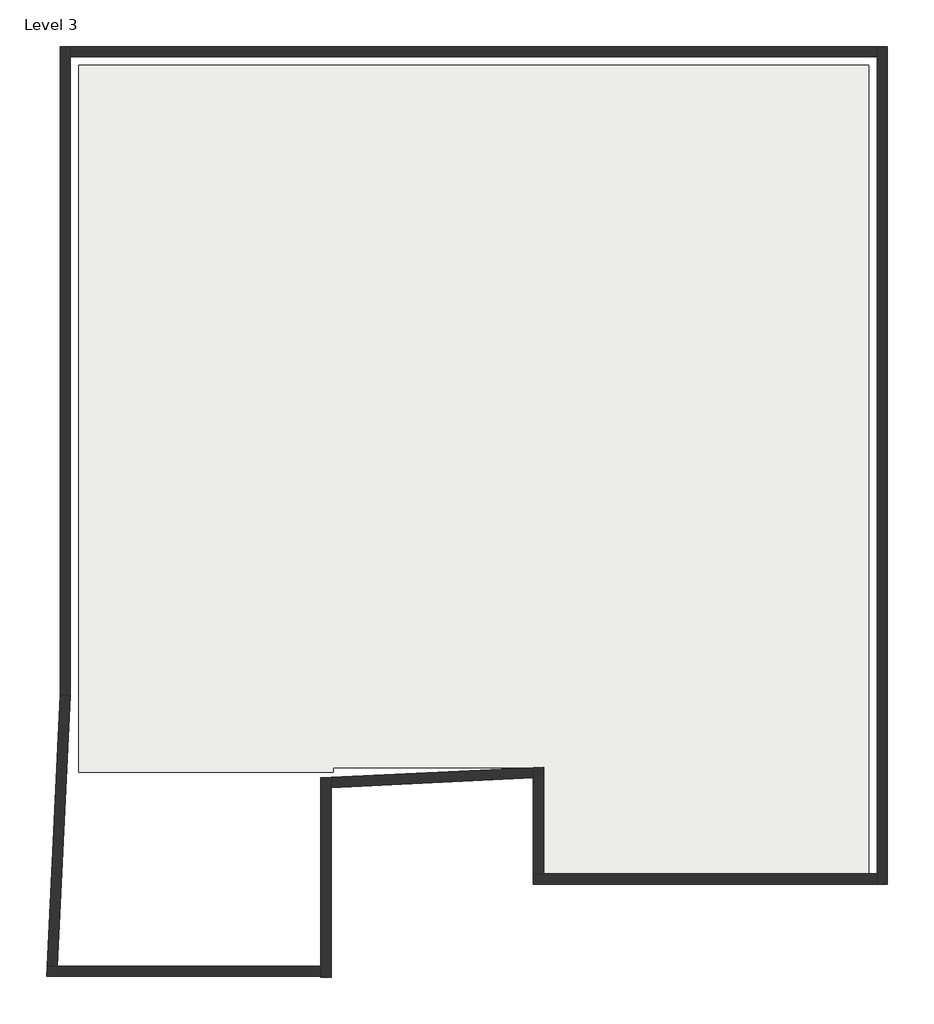
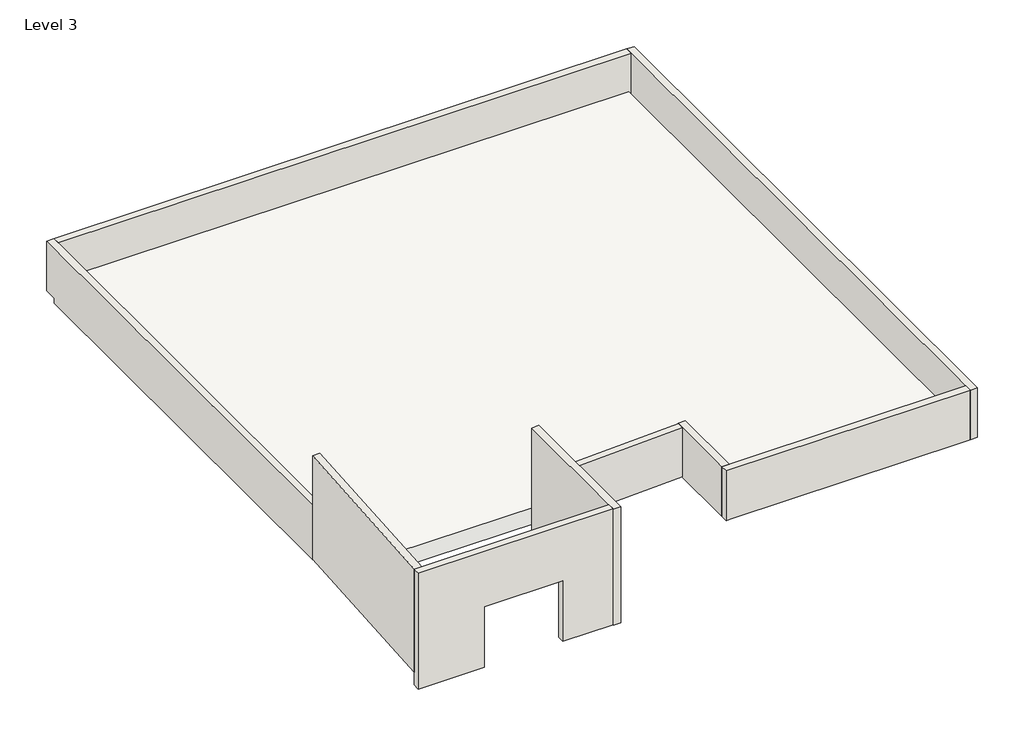
# One storey: 9 walls, 1 roof.
"""IFC4 building model written with IfcOpenShell, lengths in millimetres."""

from ifc_helpers import new_model, si_unit, frame, origin, place, context, project, spatial, polyline, outline, extrude, faceted_brep, element, save

model = new_model("IFC4")

# Units and contexts
model_context = context("Model", 3, world=origin())
ifc_project = project(units=[si_unit("LENGTHUNIT", "METRE", prefix="MILLI")], contexts=[model_context])

# Site, building, storey
site = spatial("IfcSite", under=ifc_project)
building = spatial("IfcBuilding", under=site)
storey = spatial("IfcBuildingStorey", under=building, Name="Level 3", Elevation=6400.8)

# Roof
placement = place(None, origin())
element("IfcRoof", 1, ObjectType="Generic - 12\"", at=placement, inside=storey, context=model_context, shape_type="SweptSolid", body=[
    extrude(outline(polyline([(-14760.7023867, 8292.2500137), (-4981.7023867, 8292.2500137), (-4981.7023867, -1718.5249863), (-9071.1023867, -1718.5249863), (-9071.1023867, -400.8999863), (-11611.1023867, -400.8999863), (-11611.1023867, -458.0499863), (-14760.7023867, -458.0499863), (-14760.7023867, 8292.2500137)])), frame((0.0, 0.0, 6705.6), z_axis=(0.0, 0.0, 1.0), x_axis=(1.0, 0.0, 0.0)), (0.0, 0.0, 1.0), 304.8),
])

# Walls
element("IfcWall", 2, ObjectType="INNER WALL 5\"", at=placement, inside=storey, context=model_context, shape_type="SweptSolid", body=[
    extrude(outline(polyline([(-4880.1023867, 8393.8500137), (-14863.8898867, 8393.8500137), (-14863.8898867, 8520.8500137), (-4880.1023867, 8520.8500137), (-4880.1023867, 8393.8500137)])), frame((0.0, 0.0, 6705.6), z_axis=(0.0, 0.0, 1.0), x_axis=(1.0, 0.0, 0.0)), (0.0, 0.0, 1.0), 914.4),
])
element("IfcWall", 3, ObjectType="INNER WALL 5\"", at=placement, inside=storey, context=model_context, shape_type="Brep", body=[
    faceted_brep([(-4753.1023867, -1842.3499863, 6705.6), (-4753.1023867, 8292.2500137, 6705.6), (-4753.1023867, 8520.8500137, 6705.6), (-4753.1023867, 8520.8500137, 7620.0), (-4753.1023867, -1842.3499863, 7620.0), (-4880.1023867, -1842.3499863, 6705.6), (-4880.1023867, -1842.3499863, 7620.0), (-4880.1023867, -1715.3499863, 7620.0), (-4880.1023867, 8393.8500137, 7620.0), (-4880.1023867, 8520.8500137, 7620.0), (-4880.1023867, 8520.8500137, 6705.6), (-4880.1023867, 8393.8500137, 6705.6), (-4880.1023867, -1715.3499863, 6705.6)], [[[0, 1, 2, 3, 4]], [[5, 6, 7, 8, 9, 10, 11, 12]], [[2, 1, 0, 5, 12, 11, 10]], [[4, 3, 9, 8, 7, 6]], [[3, 2, 10, 9]], [[0, 4, 6, 5]]]),
])
element("IfcWall", 4, ObjectType="INNER WALL 5\"", at=placement, inside=storey, context=model_context, shape_type="Brep", body=[
    faceted_brep([(-14990.8898867, 8292.2500137, 6618.3549278), (-14990.8898867, 492.69606, 6618.3549278), (-14990.8898867, 492.69606, 7620.0), (-14990.8898867, 8520.8500137, 7620.0), (-14990.8898867, 8520.8500137, 6705.6), (-14990.8898867, 8292.2500137, 6705.6), (-14863.8898867, 8292.2500137, 6618.3549278), (-14863.8898867, 8292.2500137, 6705.6), (-14863.8898867, 8393.8500137, 6705.6), (-14863.8898867, 8520.8500137, 6705.6), (-14863.8898867, 8520.8500137, 7620.0), (-14863.8898867, 8393.8500137, 7620.0), (-14863.8898867, 489.6542677, 7620.0), (-14863.8898867, 489.6542677, 6618.3549278)], [[[0, 1, 2, 3, 4, 5]], [[6, 7, 8, 9, 10, 11, 12, 13]], [[1, 0, 6, 13]], [[3, 2, 12, 11, 10]], [[4, 9, 8, 7, 5]], [[0, 5, 7, 6]], [[4, 3, 10, 9]], [[2, 1, 13, 12]]]),
])
element("IfcWall", 5, ObjectType="INNER WALL 5\"", at=placement, inside=storey, context=model_context, shape_type="Brep", body=[
    faceted_brep([(-11763.5023867, -2985.3499863, 8534.4), (-15157.5917172, -2985.3499863, 8534.4), (-15157.5917172, -2985.3499863, 6400.8), (-14011.4023867, -2985.3499863, 6400.8), (-14011.4023867, -2985.3499863, 7520.3640825), (-12639.8023867, -2985.3499863, 7520.3640825), (-12639.8023867, -2985.3499863, 6400.8), (-11763.5023867, -2985.3499863, 6400.8), (-15151.5046407, -2858.3499863, 8534.4), (-15024.3588484, -2858.3499863, 8534.4), (-11763.5023867, -2858.3499863, 8534.4), (-11763.5023867, -2858.3499863, 6400.8), (-12639.8023867, -2858.3499863, 6400.8), (-12639.8023867, -2858.3499863, 7520.3640825), (-14011.4023867, -2858.3499863, 7520.3640825), (-14011.4023867, -2858.3499863, 6400.8), (-15151.5046407, -2858.3499863, 6400.8), (-15151.5046407, -2858.3499863, 6630.8481004)], [[[0, 1, 2, 3, 4, 5, 6, 7]], [[8, 9, 10, 11, 12, 13, 14, 15, 16, 17]], [[11, 7, 6, 12]], [[2, 16, 15, 3]], [[1, 0, 10, 9, 8]], [[0, 7, 11, 10]], [[2, 1, 8, 17, 16]], [[5, 13, 12, 6]], [[13, 5, 4, 14]], [[14, 4, 3, 15]]]),
])
element("IfcWall", 6, ObjectType="INNER WALL 5\"", at=placement, inside=storey, context=model_context, shape_type="Brep", body=[
    faceted_brep([(-4880.1023867, -1715.3499863, 6705.6), (-4981.7023867, -1715.3499863, 6705.6), (-9007.6023867, -1715.3499863, 6705.6), (-9071.1023867, -1715.3499863, 6705.6), (-9134.6023867, -1715.3499863, 6705.6), (-9134.6023867, -1715.3499863, 7620.0), (-9007.6023867, -1715.3499863, 7620.0), (-4880.1023867, -1715.3499863, 7620.0), (-4880.1023867, -1842.3499863, 6705.6), (-4880.1023867, -1842.3499863, 7620.0), (-9134.6023867, -1842.3499863, 7620.0), (-9134.6023867, -1842.3499863, 6705.6), (-9071.1023867, -1842.3499863, 6705.6), (-4981.7023867, -1842.3499863, 6705.6)], [[[0, 1, 2, 3, 4, 5, 6, 7]], [[8, 9, 10, 11, 12, 13]], [[4, 3, 2, 1, 0, 8, 13, 12, 11]], [[7, 6, 5, 10, 9]], [[5, 4, 11, 10]], [[0, 7, 9, 8]]]),
])
element("IfcWall", 7, ObjectType="INNER WALL 5\"", at=placement, inside=storey, context=model_context, shape_type="Brep", body=[
    faceted_brep([(-9007.6023867, -1715.3499863, 6705.6), (-9007.6023867, -394.6969014, 6705.6), (-9007.6023867, -394.6969014, 7620.0), (-9007.6023867, -1715.3499863, 7620.0), (-9134.6023867, -1715.3499863, 6705.6), (-9134.6023867, -1715.3499863, 7620.0), (-9134.6023867, -400.8999863, 7620.0), (-9134.6023867, -400.8999863, 7618.4335882), (-9134.6023867, -400.8999863, 6713.109375), (-9134.6023867, -400.8999863, 6705.6)], [[[0, 1, 2, 3]], [[4, 5, 6, 7, 8, 9]], [[1, 0, 4, 9]], [[3, 2, 6, 5]], [[0, 3, 5, 4]], [[2, 1, 9, 8, 7, 6]]]),
])
element("IfcWall", 8, ObjectType="INNER WALL 5\"", at=placement, inside=storey, context=model_context, shape_type="Brep", body=[
    faceted_brep([(-11636.5023867, -2998.0499863, 6400.8), (-11636.5023867, -523.1007575, 6400.8), (-11636.5023867, -523.1007575, 6713.109375), (-11636.5023867, -523.1007575, 7618.4335882), (-11636.5023867, -523.1007575, 8534.4), (-11636.5023867, -2998.0499863, 8534.4), (-11763.5023867, -2998.0499863, 6400.8), (-11763.5023867, -2998.0499863, 8534.4), (-11763.5023867, -2985.3499863, 8534.4), (-11763.5023867, -2858.3499863, 8534.4), (-11763.5023867, -529.3038423, 8534.4), (-11763.5023867, -529.3038423, 6400.8), (-11763.5023867, -2858.3499863, 6400.8), (-11763.5023867, -2985.3499863, 6400.8)], [[[0, 1, 2, 3, 4, 5]], [[6, 7, 8, 9, 10, 11, 12, 13]], [[1, 0, 6, 13, 12, 11]], [[5, 4, 10, 9, 8, 7]], [[0, 5, 7, 6]], [[4, 3, 2, 1, 11, 10]]]),
])
element("IfcWall", 9, ObjectType="INNER WALL 5\"", at=placement, inside=storey, context=model_context, shape_type="SweptSolid", body=[
    extrude(outline(polyline([(-14863.8898867, 489.6542677), (-15024.3588484, -2858.3499863), (-15151.5046407, -2858.3499863), (-14990.8898867, 492.69606), (-14863.8898867, 489.6542677)])), frame((0.0, 0.0, 6630.8481004), z_axis=(0.0, 0.0, 1.0), x_axis=(1.0, 0.0, 0.0)), (0.0, 0.0, 1.0), 1903.5518996),
])
element("IfcWall", 10, ObjectType="INNER WALL 5\"", at=placement, inside=storey, context=model_context, shape_type="SweptSolid", body=[
    extrude(outline(polyline([(-9134.6023867, -528.0513852), (-11636.5023867, -650.2521564), (-11636.5023867, -523.1007575), (-9134.6023867, -400.8999863), (-9134.6023867, -528.0513852)])), frame((0.0, 0.0, 6713.109375), z_axis=(0.0, 0.0, 1.0), x_axis=(1.0, 0.0, 0.0)), (0.0, 0.0, 1.0), 905.3242132),
])

save(model, "model.ifc")

# Revit data of these elements
# Type "Generic - 12\""
#   Assembly Code = "B1020"
#   Layers, outside or top first: 1' - 0" no material (function 1)
# Type "INNER WALL 5\""
#   Assembly Code = "B2010"
#   Layers, outside or top first: 0' - 5" "OUTER WALL" (function 1)
# Element 1 (IfcRoof, "Generic - 12\"")
#   built-in parameter 1001705 = 23 (stored number, unit not read)
#   built-in parameter 1001701 = 1 (stored number, unit not read)
#   built-in parameter 1001710 = 33615
#   Phase Created = New Construction
#   Materials on its faces: "Default Roof"
# Elements 2, 3, 6, 7 (IfcWall, "INNER WALL 5\"")
#   built-in parameter 1001111 = 1' - 0"
#   Top Offset = 0' - 0"
#   Base Offset = 1' - 0"
#   Unconnected Height = 3' - 0"
#   wall height = 3' - 0"
#   Phase Created = New Construction
#   Base Constraint = Level 3
#   Materials on its faces: "OUTER WALL"
# Element 4 (IfcWall, "INNER WALL 5\"")
#   built-in parameter 1001111 = 0' - 8.56515"
#   Top Offset = 0' - 0"
#   Base Offset = 0' - 8.56515"
#   Unconnected Height = 3' - 3.43485"
#   wall height = 3' - 3.43485"
#   Phase Created = New Construction
#   Base Constraint = Level 3
#   Materials on its faces: "OUTER WALL"
# Elements 5, 8 (IfcWall, "INNER WALL 5\"")
#   Top Offset = 0' - 0"
#   Base Offset = 0' - 0"
#   Unconnected Height = 7' - 0"
#   wall height = 7' - 0"
#   Phase Created = New Construction
#   Base Constraint = Level 3
#   Materials on its faces: "OUTER WALL"
# Element 9 (IfcWall, "INNER WALL 5\"")
#   built-in parameter 1001111 = 0' - 9.05701"
#   Top Offset = 0' - 0"
#   Base Offset = 0' - 9.05701"
#   Unconnected Height = 6' - 2.94299"
#   wall height = 6' - 2.94299"
#   Phase Created = New Construction
#   Base Constraint = Level 3
#   Materials on its faces: "OUTER WALL"
# Element 10 (IfcWall, "INNER WALL 5\"")
#   built-in parameter 1001111 = 1' - 0.29564"
#   Top Offset = 0' - 0"
#   Base Offset = 1' - 0.29564"
#   Unconnected Height = 2' - 11.64269"
#   wall height = 2' - 11.64269"
#   Phase Created = New Construction
#   Base Constraint = Level 3
#   Materials on its faces: "OUTER WALL"
# Materials
#   "OUTER WALL": class "Generic", colour RGB 245 245 240, transparency 0, Cost = 0
#   "Default Roof": colour RGB 88 101 114, transparency 0, Cost = 0
